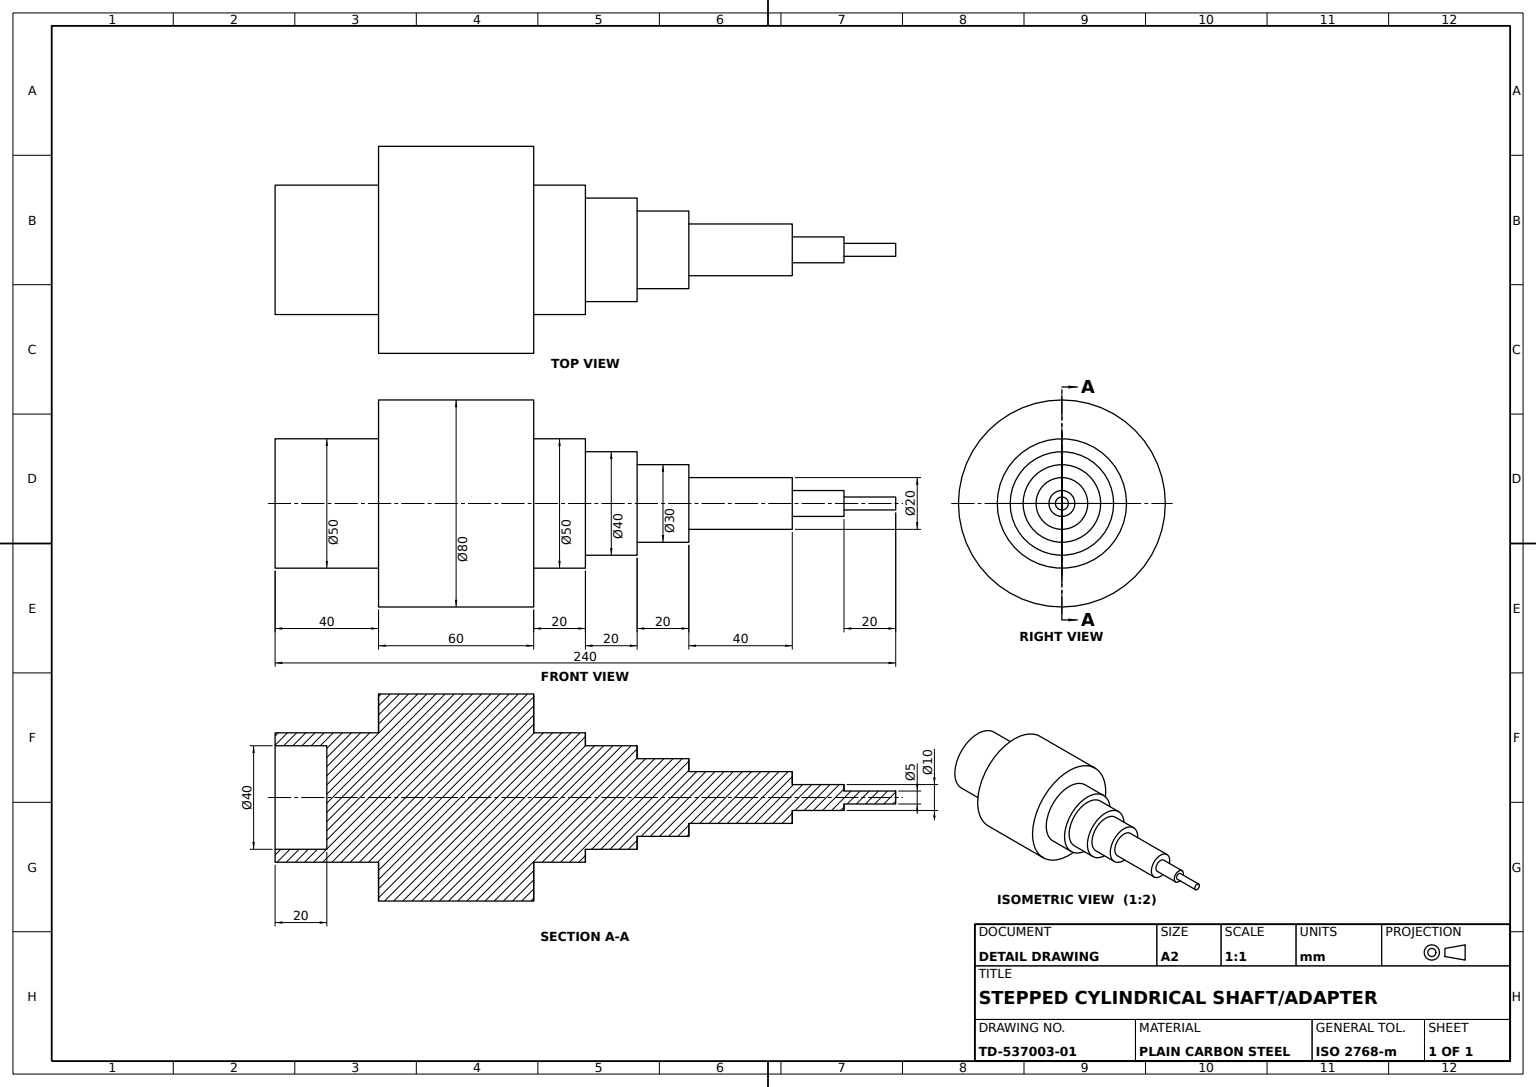
from build123d import *

# Parameters (mm, degrees)
COLLAR_PROFILE_80_R     = 40
COLLAR_80_DEPTH         = 60
SPIGOT_SKETCH_50_R      = 25
SPIGOT_50_DEPTH         = 40
SPIGOT_BORE_SKETCH_40_R = 20
SPIGOT_BORE_40_DEPTH    = 20
PIN_START               = 20
PIN_STEP_1_SKETCH_50_R  = 25
PIN_STEP_1_50_DEPTH     = 20
PIN_STEP_2_SKETCH_40_R  = 20
PIN_STEP_2_40_DEPTH     = 20
PIN_STEP_3_SKETCH_30_R  = 15
PIN_STEP_3_30_DEPTH     = 20
PIN_STEP_4_SKETCH_20_R  = 10
PIN_STEP_4_20_DEPTH     = 20
PIN_STEP_5_SKETCH_20_R  = 10
PIN_STEP_5_20_DEPTH     = 20
PIN_STEP_6_SKETCH_10_R  = 5
PIN_STEP_6_10_DEPTH     = 20
PIN_TIP_SKETCH_5_R      = 2.5
PIN_TIP_5_DEPTH         = 20


with BuildPart() as part:
    # Collar Profile Ø80 → Collar Ø80 (new body)
    with BuildSketch(Plane.XY):
        Circle(COLLAR_PROFILE_80_R)
    extrude(amount=COLLAR_80_DEPTH)

    # Spigot Sketch Ø50 → Spigot Ø50 (add)
    with BuildSketch(Plane.XY.offset(60)):
        Circle(SPIGOT_SKETCH_50_R)
    extrude(amount=SPIGOT_50_DEPTH)

    # Spigot Bore Sketch Ø40 → Spigot Bore Ø40 (cut)
    with BuildSketch(Plane.XY.offset(100)):
        Circle(SPIGOT_BORE_SKETCH_40_R)
    extrude(amount=-SPIGOT_BORE_40_DEPTH, mode=Mode.SUBTRACT)

    # Pin Step 1 Sketch Ø50 → Pin Step 1 Ø50 (add)
    with BuildSketch(Plane(origin=(0, 0, 0), x_dir=(-1, 0, 0), z_dir=(0, 0, -1)).offset(PIN_START)):
        with Locations(Location((0, 0, 0), (0, 0, 180))):
            Circle(PIN_STEP_1_SKETCH_50_R)
    extrude(amount=-PIN_STEP_1_50_DEPTH)

    # Pin Step 2 Sketch Ø40 → Pin Step 2 Ø40 (add)
    with BuildSketch(Plane(origin=(0, 0, -20), x_dir=(-1, 0, 0), z_dir=(0, 0, -1))):
        with Locations(Location((0, 0, 0), (0, 0, 180))):
            Circle(PIN_STEP_2_SKETCH_40_R)
    extrude(amount=PIN_STEP_2_40_DEPTH)

    # Pin Step 3 Sketch Ø30 → Pin Step 3 Ø30 (add)
    with BuildSketch(Plane(origin=(0, 0, -40), x_dir=(-1, 0, 0), z_dir=(0, 0, -1))):
        Circle(PIN_STEP_3_SKETCH_30_R)
    extrude(amount=PIN_STEP_3_30_DEPTH)

    # Pin Step 4 Sketch Ø20 → Pin Step 4 Ø20 (add)
    with BuildSketch(Plane(origin=(0, 0, -60), x_dir=(-1, 0, 0), z_dir=(0, 0, -1))):
        Circle(PIN_STEP_4_SKETCH_20_R)
    extrude(amount=PIN_STEP_4_20_DEPTH)

    # Pin Step 5 Sketch Ø20 → Pin Step 5 Ø20 (add)
    with BuildSketch(Plane(origin=(0, 0, -80), x_dir=(-1, 0, 0), z_dir=(0, 0, -1))):
        Circle(PIN_STEP_5_SKETCH_20_R)
    extrude(amount=PIN_STEP_5_20_DEPTH)

    # Pin Step 6 Sketch Ø10 → Pin Step 6 Ø10 (add)
    with BuildSketch(Plane(origin=(0, 0, -100), x_dir=(-1, 0, 0), z_dir=(0, 0, -1))):
        Circle(PIN_STEP_6_SKETCH_10_R)
    extrude(amount=PIN_STEP_6_10_DEPTH)

    # Pin Tip Sketch Ø5 → Pin Tip Ø5 (add)
    with BuildSketch(Plane(origin=(0, 0, -120), x_dir=(-1, 0, 0), z_dir=(0, 0, -1))):
        Circle(PIN_TIP_SKETCH_5_R)
    extrude(amount=PIN_TIP_5_DEPTH)


solid = part.part
